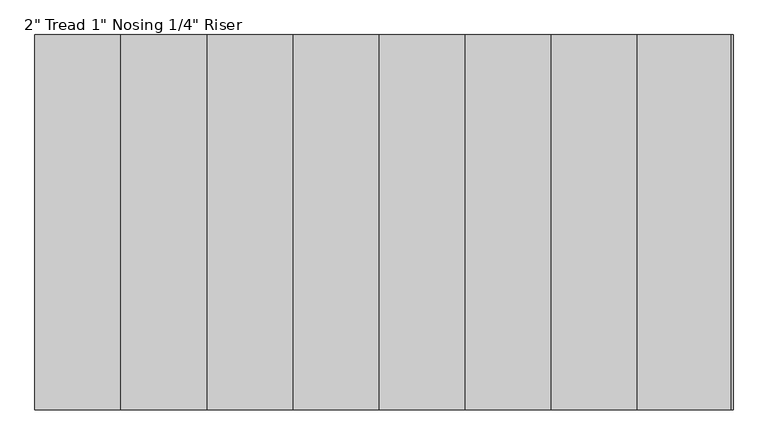
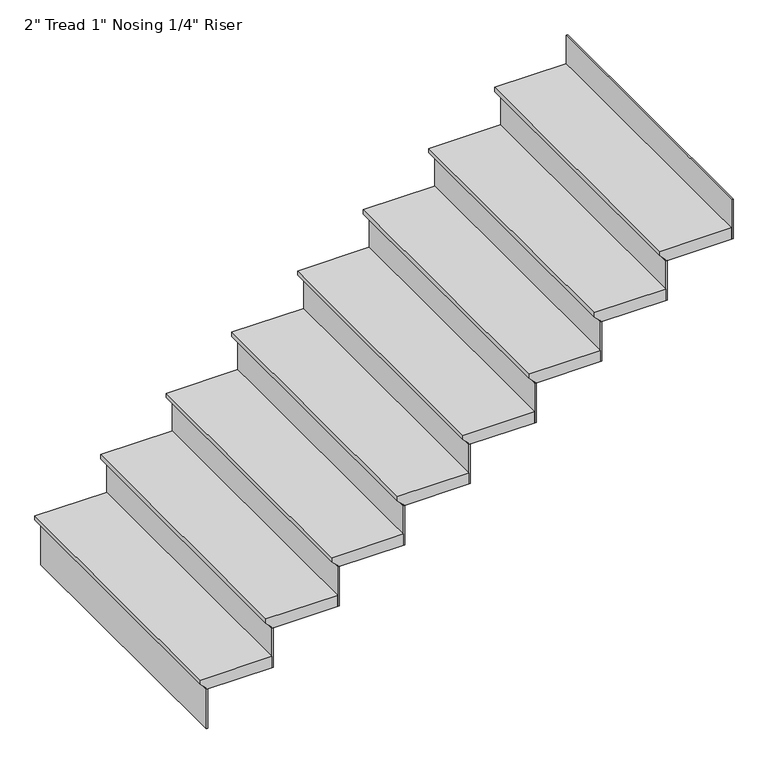
"""IFC4 building model written with IfcOpenShell, lengths in millimetres: stair flight geometry."""

from ifc_helpers import new_model, si_unit, frame, origin, place, context, project, spatial, polyline, outline, extrude, source, transform, mapped, element, save


def stair_flight_057ca7f5(model_context):
    return source(origin(), model_context, "Body", "SweptSolid", [
        extrude(outline(polyline([(1778.0, -7819.2791271), (1778.0, -8124.0791271), (1758.95, -8124.0791271), (1733.55, -8098.6791271), (1727.2, -8098.6791271), (1727.2, -7819.2791271), (1778.0, -7819.2791271)])), frame((0.0, 6461.9953048, 0.0), z_axis=(0.0, 1.0, 0.0), x_axis=(0.0, 0.0, 1.0)), (0.0, 0.0, 1.0), 1219.2),
        extrude(outline(polyline([(-8092.3291271, 6461.9953048), (-8098.6791271, 6461.9953048), (-8098.6791271, 7681.1953048), (-8092.3291271, 7681.1953048), (-8092.3291271, 6461.9953048)])), frame((0.0, 0.0, 1549.4), z_axis=(0.0, 0.0, 1.0), x_axis=(1.0, 0.0, 0.0)), (0.0, 0.0, 1.0), 177.8),
        extrude(outline(polyline([(-7812.9291271, 6461.9953048), (-7819.2791271, 6461.9953048), (-7819.2791271, 7681.1953048), (-7812.9291271, 7681.1953048), (-7812.9291271, 6461.9953048)])), frame((0.0, 0.0, 1727.2), z_axis=(0.0, 0.0, 1.0), x_axis=(1.0, 0.0, 0.0)), (0.0, 0.0, 1.0), 177.8),
        extrude(outline(polyline([(1955.8, -7539.8791271), (1955.8, -7844.6791271), (1936.75, -7844.6791271), (1911.35, -7819.2791271), (1905.0, -7819.2791271), (1905.0, -7539.8791271), (1955.8, -7539.8791271)])), frame((0.0, 6461.9953048, 0.0), z_axis=(0.0, 1.0, 0.0), x_axis=(0.0, 0.0, 1.0)), (0.0, 0.0, 1.0), 1219.2),
        extrude(outline(polyline([(-7533.5291271, 6461.9953048), (-7539.8791271, 6461.9953048), (-7539.8791271, 7681.1953048), (-7533.5291271, 7681.1953048), (-7533.5291271, 6461.9953048)])), frame((0.0, 0.0, 1905.0), z_axis=(0.0, 0.0, 1.0), x_axis=(1.0, 0.0, 0.0)), (0.0, 0.0, 1.0), 177.8),
        extrude(outline(polyline([(2133.6, -7260.4791271), (2133.6, -7565.2791271), (2114.55, -7565.2791271), (2089.15, -7539.8791271), (2082.8, -7539.8791271), (2082.8, -7260.4791271), (2133.6, -7260.4791271)])), frame((0.0, 6461.9953048, 0.0), z_axis=(0.0, 1.0, 0.0), x_axis=(0.0, 0.0, 1.0)), (0.0, 0.0, 1.0), 1219.2),
        extrude(outline(polyline([(-7254.1291271, 6461.9953048), (-7260.4791271, 6461.9953048), (-7260.4791271, 7681.1953048), (-7254.1291271, 7681.1953048), (-7254.1291271, 6461.9953048)])), frame((0.0, 0.0, 2082.8), z_axis=(0.0, 0.0, 1.0), x_axis=(1.0, 0.0, 0.0)), (0.0, 0.0, 1.0), 177.8),
        extrude(outline(polyline([(2311.4, -6981.0791271), (2311.4, -7285.8791271), (2292.35, -7285.8791271), (2266.95, -7260.4791271), (2260.6, -7260.4791271), (2260.6, -6981.0791271), (2311.4, -6981.0791271)])), frame((0.0, 6461.9953048, 0.0), z_axis=(0.0, 1.0, 0.0), x_axis=(0.0, 0.0, 1.0)), (0.0, 0.0, 1.0), 1219.2),
        extrude(outline(polyline([(-6974.7291271, 6461.9953048), (-6981.0791271, 6461.9953048), (-6981.0791271, 7681.1953048), (-6974.7291271, 7681.1953048), (-6974.7291271, 6461.9953048)])), frame((0.0, 0.0, 2260.6), z_axis=(0.0, 0.0, 1.0), x_axis=(1.0, 0.0, 0.0)), (0.0, 0.0, 1.0), 177.8),
        extrude(outline(polyline([(2489.2, -6701.6791271), (2489.2, -7006.4791271), (2470.15, -7006.4791271), (2444.75, -6981.0791271), (2438.4, -6981.0791271), (2438.4, -6701.6791271), (2489.2, -6701.6791271)])), frame((0.0, 6461.9953048, 0.0), z_axis=(0.0, 1.0, 0.0), x_axis=(0.0, 0.0, 1.0)), (0.0, 0.0, 1.0), 1219.2),
        extrude(outline(polyline([(-6695.3291271, 6461.9953048), (-6701.6791271, 6461.9953048), (-6701.6791271, 7681.1953048), (-6695.3291271, 7681.1953048), (-6695.3291271, 6461.9953048)])), frame((0.0, 0.0, 2438.4), z_axis=(0.0, 0.0, 1.0), x_axis=(1.0, 0.0, 0.0)), (0.0, 0.0, 1.0), 177.8),
        extrude(outline(polyline([(2667.0, -6422.2791271), (2667.0, -6727.0791271), (2647.95, -6727.0791271), (2622.55, -6701.6791271), (2616.2, -6701.6791271), (2616.2, -6422.2791271), (2667.0, -6422.2791271)])), frame((0.0, 6461.9953048, 0.0), z_axis=(0.0, 1.0, 0.0), x_axis=(0.0, 0.0, 1.0)), (0.0, 0.0, 1.0), 1219.2),
        extrude(outline(polyline([(-6415.9291271, 6461.9953048), (-6422.2791271, 6461.9953048), (-6422.2791271, 7681.1953048), (-6415.9291271, 7681.1953048), (-6415.9291271, 6461.9953048)])), frame((0.0, 0.0, 2616.2), z_axis=(0.0, 0.0, 1.0), x_axis=(1.0, 0.0, 0.0)), (0.0, 0.0, 1.0), 177.8),
        extrude(outline(polyline([(2844.8, -6142.8791271), (2844.8, -6447.6791271), (2825.75, -6447.6791271), (2800.35, -6422.2791271), (2794.0, -6422.2791271), (2794.0, -6142.8791271), (2844.8, -6142.8791271)])), frame((0.0, 6461.9953048, 0.0), z_axis=(0.0, 1.0, 0.0), x_axis=(0.0, 0.0, 1.0)), (0.0, 0.0, 1.0), 1219.2),
        extrude(outline(polyline([(-6136.5291271, 6461.9953048), (-6142.8791271, 6461.9953048), (-6142.8791271, 7681.1953048), (-6136.5291271, 7681.1953048), (-6136.5291271, 6461.9953048)])), frame((0.0, 0.0, 2794.0), z_axis=(0.0, 0.0, 1.0), x_axis=(1.0, 0.0, 0.0)), (0.0, 0.0, 1.0), 177.8),
        extrude(outline(polyline([(-5857.1291271, 6461.9953048), (-5863.4791271, 6461.9953048), (-5863.4791271, 7681.1953048), (-5857.1291271, 7681.1953048), (-5857.1291271, 6461.9953048)])), frame((0.0, 0.0, 2971.8), z_axis=(0.0, 0.0, 1.0), x_axis=(1.0, 0.0, 0.0)), (0.0, 0.0, 1.0), 177.8),
        extrude(outline(polyline([(3022.6, -5863.4791271), (3022.6, -6168.2791271), (3003.55, -6168.2791271), (2978.15, -6142.8791271), (2971.8, -6142.8791271), (2971.8, -5863.4791271), (3022.6, -5863.4791271)])), frame((0.0, 6461.9953048, 0.0), z_axis=(0.0, 1.0, 0.0), x_axis=(0.0, 0.0, 1.0)), (0.0, 0.0, 1.0), 1219.2),
    ])


if __name__ == "__main__":
    model = new_model("IFC4")
    model_context = context("Model", 3, world=origin())
    ifc_project = project(units=[si_unit("LENGTHUNIT", "METRE", prefix="MILLI")], contexts=[model_context])
    site = spatial("IfcSite", under=ifc_project)
    building = spatial("IfcBuilding", under=site)
    placement = place(None, origin())
    stair_flight_shape = stair_flight_057ca7f5(model_context)
    element("IfcStairFlight", 1, ObjectType="2\" Tread 1\" Nosing 1/4\" Riser", at=placement, inside=building, context=model_context, shape_type="MappedRepresentation", body=[
        mapped(stair_flight_shape, transform((0.0, 0.0, 0.0), x_axis=(1.0, 0.0, 0.0), y_axis=(0.0, 1.0, 0.0), z_axis=(0.0, 0.0, 1.0))),
    ])
    save(model, "model.ifc")
